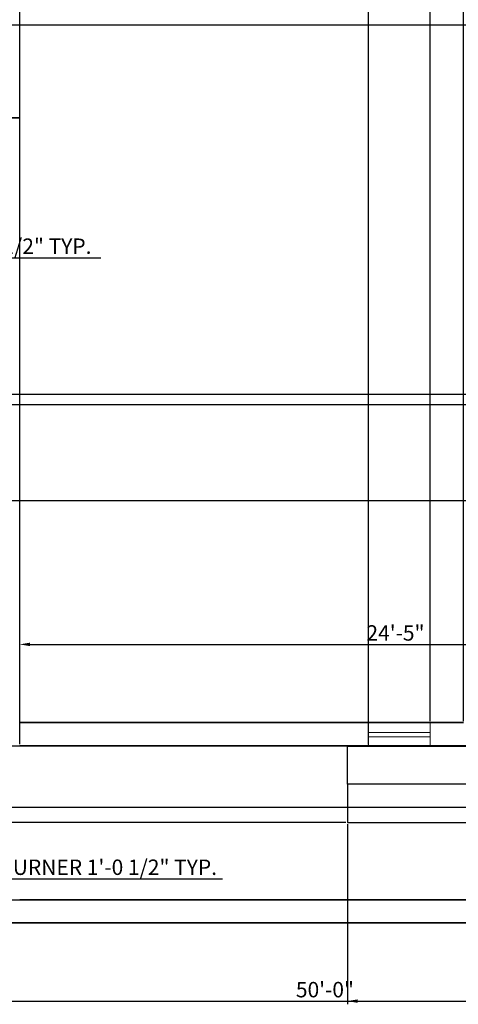
# Model space of a CAD drawing. Units: inches. Extents: x 1973 to 2661, y 1730 to 2412.
# Tile 2 of 5: x 2197 to 2368, y 1734 to 2117. Entities that reach past the tile are written whole.
import ezdxf

# ---------------------------------------------------------------- set-up
doc = ezdxf.new("R2010")
doc.units = ezdxf.units.IN
for name, color, linetype, lineweight in [('A-ANNO-DIMS', 2, 'Continuous', 18), ('A-FLOR-STRS', 7, 'Continuous', 25), ('A-GLAZ', 4, 'Continuous', 18), ('A-WALL', 7, 'Continuous', 35)]:
    doc.layers.add(name, color=color, linetype=linetype, lineweight=lineweight)
doc.styles.get("Standard").update_dxf_attribs({"font": 'arial.ttf'})
doc.dimstyles.new('ISO-25', dxfattribs={"dimtxt": 6, "dimasz": 4, "dimexe": 1.25, "dimexo": 0.625, "dimtad": 1, "dimdec": 0, "dimrnd": 6, "dimlunit": 3, "dimtxsty": 'Standard', "dimcen": 2.5, "dimadec": 0, "dimazin": 0, "dimtfac": 1, "dimtdec": 0, "dimtmove": 0, "dimatfit": 3, "dimfxl": 1, "dimarcsym": 0})

# ---------------------------------------------------------------- blocks, each defined once
blk = doc.blocks.new('*D16')
at = {"layer": 'A-ANNO-DIMS', "color": 0, "lineweight": -2, "transparency": 16777216}
for p, q in [((2092.18, 2025.82), (2092.18, 2023.31)), ((2096.18, 2024.56), (2100.77, 2024.56)), ((2104.77, 2025.82), (2104.77, 2023.31)), ((2104.77, 2024.56), (2228.74, 2024.56))]:
    blk.add_line(p, q, dxfattribs=at)
at = {"layer": 'A-ANNO-DIMS', "color": 0, "transparency": 16777216}
for points in [[(2096.18, 2025.23), (2096.18, 2023.89), (2092.18, 2024.56)], [(2100.77, 2025.23), (2100.77, 2023.89), (2104.77, 2024.56)]]:
    blk.add_solid(points, dxfattribs=at)
at = {"layer": 'Defpoints', "color": 0, "transparency": 16777216}
for p in [(2092.18, 2026.45), (2104.77, 2026.45), (2104.77, 2024.56)]:
    blk.add_point(p, dxfattribs=at)
at = {"layer": 'A-ANNO-DIMS', "color": 0, "transparency": 16777216, "insert": (2168.76, 2028.29), "char_height": 6, "attachment_point": 5}
blk.add_mtext('PLACE SETTING 1\'-0 1/2" TYP.', dxfattribs=at)
blk = doc.blocks.new('*D28')
at = {"layer": 'A-ANNO-DIMS', "color": 0, "lineweight": -2, "transparency": 16777216}
for p, q in [((2170.36, 1783.74), (2170.36, 1781.24)), ((2174.36, 1782.49), (2178.84, 1782.49)), ((2182.84, 1783.74), (2182.84, 1781.24)), ((2182.84, 1782.49), (2276.1, 1782.49))]:
    blk.add_line(p, q, dxfattribs=at)
at = {"layer": 'A-ANNO-DIMS', "color": 0, "transparency": 16777216}
for points in [[(2174.36, 1783.16), (2174.36, 1781.83), (2170.36, 1782.49)], [(2178.84, 1783.16), (2178.84, 1781.83), (2182.84, 1782.49)]]:
    blk.add_solid(points, dxfattribs=at)
at = {"layer": 'Defpoints', "color": 0, "transparency": 16777216}
for p in [(2170.36, 1784.36), (2182.84, 1784.36), (2182.84, 1782.49)]:
    blk.add_point(p, dxfattribs=at)
at = {"layer": 'A-ANNO-DIMS', "color": 0, "transparency": 16777216, "insert": (2231.47, 1786.22), "char_height": 6, "attachment_point": 5}
blk.add_mtext('BURNER 1\'-0 1/2" TYP.', dxfattribs=at)
blk = doc.blocks.new('*D30')
at = {"layer": 'A-ANNO-DIMS', "color": 0, "lineweight": -2, "transparency": 16777216}
for p, q in [((2016.04, 1764.73), (2016.04, 1733.57)), ((2616.04, 1764.73), (2616.04, 1733.57)), ((2020.04, 1734.82), (2612.04, 1734.82))]:
    blk.add_line(p, q, dxfattribs=at)
at = {"layer": 'A-ANNO-DIMS', "color": 0, "transparency": 16777216}
for points in [[(2020.04, 1735.49), (2020.04, 1734.15), (2016.04, 1734.82)], [(2612.04, 1735.49), (2612.04, 1734.15), (2616.04, 1734.82)]]:
    blk.add_solid(points, dxfattribs=at)
at = {"layer": 'Defpoints', "color": 0, "transparency": 16777216}
for p in [(2016.04, 1765.35), (2616.04, 1765.35), (2616.04, 1734.82)]:
    blk.add_point(p, dxfattribs=at)
at = {"layer": 'A-ANNO-DIMS', "color": 0, "transparency": 16777216, "insert": (2316.04, 1738.51), "char_height": 6, "attachment_point": 5}
blk.add_mtext('50\'-0"', dxfattribs=at)
blk = doc.blocks.new('*D53')
at = {"layer": 'A-ANNO-DIMS', "color": 0, "lineweight": -2, "transparency": 16777216}
for p, q in [((2197.04, 1843.98), (2197.04, 1875.1)), ((2201.04, 1873.85), (2486.04, 1873.85)), ((2490.04, 1843.98), (2490.04, 1875.1))]:
    blk.add_line(p, q, dxfattribs=at)
at = {"layer": 'A-ANNO-DIMS', "color": 0, "transparency": 16777216}
for points in [[(2201.04, 1874.52), (2201.04, 1873.18), (2197.04, 1873.85)], [(2486.04, 1874.52), (2486.04, 1873.18), (2490.04, 1873.85)]]:
    blk.add_solid(points, dxfattribs=at)
at = {"layer": 'Defpoints', "color": 0, "transparency": 16777216}
for p in [(2490.04, 1873.85), (2197.04, 1843.35), (2490.04, 1843.35)]:
    blk.add_point(p, dxfattribs=at)
at = {"layer": 'A-ANNO-DIMS', "color": 0, "transparency": 16777216, "insert": (2343.54, 1877.54), "char_height": 6, "attachment_point": 5}
blk.add_mtext('24\'-5"', dxfattribs=at)
blk = doc.blocks.new('*D54')
at = {"layer": 'A-ANNO-DIMS', "color": 0, "lineweight": -2, "transparency": 16777216}
for p, q in [((2197.04, 1834.98), (2197.04, 2397.1)), ((2201.04, 2395.85), (2329.03, 2395.85)), ((2333.03, 1834.87), (2333.03, 2397.1))]:
    blk.add_line(p, q, dxfattribs=at)
at = {"layer": 'A-ANNO-DIMS', "color": 0, "transparency": 16777216}
for points in [[(2201.04, 2396.52), (2201.04, 2395.18), (2197.04, 2395.85)], [(2329.03, 2396.52), (2329.03, 2395.18), (2333.03, 2395.85)]]:
    blk.add_solid(points, dxfattribs=at)
at = {"layer": 'Defpoints', "color": 0, "transparency": 16777216}
for p in [(2333.03, 2395.85), (2197.04, 1834.35), (2333.03, 1834.25)]:
    blk.add_point(p, dxfattribs=at)
at = {"layer": 'A-ANNO-DIMS', "color": 0, "transparency": 16777216, "insert": (2265.03, 2399.49), "char_height": 6, "attachment_point": 5}
blk.add_mtext('11\'-4"', dxfattribs=at)
blk = doc.blocks.new('*D57')
at = {"layer": 'A-ANNO-DIMS', "color": 0, "lineweight": -2, "transparency": 16777216}
for p, q in [((2193.67, 1810.35), (2647.79, 1810.35)), ((2646.54, 1778.35), (2646.54, 1806.35)), ((2193.67, 1774.35), (2647.79, 1774.35))]:
    blk.add_line(p, q, dxfattribs=at)
at = {"layer": 'A-ANNO-DIMS', "color": 0, "transparency": 16777216}
for points in [[(2645.88, 1806.35), (2647.21, 1806.35), (2646.54, 1810.35)], [(2645.88, 1778.35), (2647.21, 1778.35), (2646.54, 1774.35)]]:
    blk.add_solid(points, dxfattribs=at)
at = {"layer": 'Defpoints', "color": 0, "transparency": 16777216}
for p in [(2193.04, 1810.35), (2646.54, 1810.35), (2193.04, 1774.35)]:
    blk.add_point(p, dxfattribs=at)
at = {"layer": 'A-ANNO-DIMS', "color": 0, "transparency": 16777216, "insert": (2642.85, 1792.35), "char_height": 6, "attachment_point": 5, "rotation": 90}
blk.add_mtext('3\'-0"', dxfattribs=at)
blk = doc.blocks.new('*D59')
at = {"layer": 'A-ANNO-DIMS', "color": 0, "lineweight": -2, "transparency": 16777216}
for p, q in [((2193.67, 2115.35), (2647.79, 2115.35)), ((2646.54, 1975.35), (2646.54, 2111.35)), ((2193.67, 1971.35), (2647.79, 1971.35))]:
    blk.add_line(p, q, dxfattribs=at)
at = {"layer": 'A-ANNO-DIMS', "color": 0, "transparency": 16777216}
for points in [[(2645.88, 2111.35), (2647.21, 2111.35), (2646.54, 2115.35)], [(2645.88, 1975.35), (2647.21, 1975.35), (2646.54, 1971.35)]]:
    blk.add_solid(points, dxfattribs=at)
at = {"layer": 'Defpoints', "color": 0, "transparency": 16777216}
for p in [(2193.04, 2115.35), (2646.54, 2115.35), (2193.04, 1971.35)]:
    blk.add_point(p, dxfattribs=at)
at = {"layer": 'A-ANNO-DIMS', "color": 0, "transparency": 16777216, "insert": (2642.85, 2043.35), "char_height": 6, "attachment_point": 5, "rotation": 90}
blk.add_mtext('12\'-0"', dxfattribs=at)
blk = doc.blocks.new('*D64')
at = {"layer": 'A-ANNO-DIMS', "color": 0, "lineweight": -2, "transparency": 16777216}
for p, q in [((2324.17, 1834.25), (1984.22, 1834.25)), ((1985.47, 1808.45), (1985.47, 1830.25)), ((2324.17, 1804.45), (1984.22, 1804.45))]:
    blk.add_line(p, q, dxfattribs=at)
at = {"layer": 'A-ANNO-DIMS', "color": 0, "transparency": 16777216}
for points in [[(1984.81, 1830.25), (1986.14, 1830.25), (1985.47, 1834.25)], [(1984.81, 1808.45), (1986.14, 1808.45), (1985.47, 1804.45)]]:
    blk.add_solid(points, dxfattribs=at)
at = {"layer": 'Defpoints', "color": 0, "transparency": 16777216}
for p in [(1985.47, 1834.25), (2324.79, 1834.25), (2324.79, 1804.45)]:
    blk.add_point(p, dxfattribs=at)
at = {"layer": 'A-ANNO-DIMS', "color": 0, "transparency": 16777216, "insert": (1981.79, 1819.35), "char_height": 6, "attachment_point": 5, "rotation": 90}
blk.add_mtext('2\'-6"', dxfattribs=at)
blk = doc.blocks.new('*D65')
at = {"layer": 'A-ANNO-DIMS', "color": 0, "lineweight": -2, "transparency": 16777216}
for p, q in [((2324.79, 1803.83), (2324.79, 1733.57)), ((2485.69, 1803.83), (2485.69, 1733.57)), ((2328.79, 1734.82), (2481.69, 1734.82))]:
    blk.add_line(p, q, dxfattribs=at)
at = {"layer": 'A-ANNO-DIMS', "color": 0, "transparency": 16777216}
for points in [[(2328.79, 1735.49), (2328.79, 1734.15), (2324.79, 1734.82)], [(2481.69, 1735.49), (2481.69, 1734.15), (2485.69, 1734.82)]]:
    blk.add_solid(points, dxfattribs=at)
at = {"layer": 'Defpoints', "color": 0, "transparency": 16777216}
for p in [(2324.79, 1804.45), (2485.69, 1804.45), (2485.69, 1734.82)]:
    blk.add_point(p, dxfattribs=at)
at = {"layer": 'A-ANNO-DIMS', "color": 0, "transparency": 16777216, "insert": (2405.24, 1738.51), "char_height": 6, "attachment_point": 5}
blk.add_mtext('13\'-5"', dxfattribs=at)
blk = doc.blocks.new('*D66')
at = {"layer": 'A-ANNO-DIMS', "color": 0, "lineweight": -2, "transparency": 16777216}
for p, q in [((2333.03, 1843.98), (2333.03, 2397.1)), ((2337.03, 2395.85), (2353.02, 2395.85)), ((2357.02, 1843.98), (2357.02, 2397.1))]:
    blk.add_line(p, q, dxfattribs=at)
at = {"layer": 'A-ANNO-DIMS', "color": 0, "transparency": 16777216}
for points in [[(2337.03, 2396.52), (2337.03, 2395.18), (2333.03, 2395.85)], [(2353.02, 2396.52), (2353.02, 2395.18), (2357.02, 2395.85)]]:
    blk.add_solid(points, dxfattribs=at)
at = {"layer": 'Defpoints', "color": 0, "transparency": 16777216}
for p in [(2357.02, 2395.85), (2333.03, 1843.35), (2357.02, 1843.35)]:
    blk.add_point(p, dxfattribs=at)
at = {"layer": 'A-ANNO-DIMS', "color": 0, "transparency": 16777216, "insert": (2345.02, 2399.54), "char_height": 6, "attachment_point": 5}
blk.add_mtext('2\'-0"', dxfattribs=at)
blk = doc.blocks.new('*D69')
at = {"layer": 'A-ANNO-DIMS', "color": 0, "lineweight": -2, "transparency": 16777216}
for p, q in [((2357.02, 1843.98), (2357.02, 2397.1)), ((2361.02, 2395.85), (2366.04, 2395.85)), ((2370.04, 1843.98), (2370.04, 2397.1)), ((2370.04, 2395.85), (2390.68, 2395.85))]:
    blk.add_line(p, q, dxfattribs=at)
at = {"layer": 'A-ANNO-DIMS', "color": 0, "transparency": 16777216}
for points in [[(2361.02, 2396.52), (2361.02, 2395.18), (2357.02, 2395.85)], [(2366.04, 2396.52), (2366.04, 2395.18), (2370.04, 2395.85)]]:
    blk.add_solid(points, dxfattribs=at)
at = {"layer": 'Defpoints', "color": 0, "transparency": 16777216}
for p in [(2370.04, 2395.85), (2357.02, 1843.35), (2370.04, 1843.35)]:
    blk.add_point(p, dxfattribs=at)
at = {"layer": 'A-ANNO-DIMS', "color": 0, "transparency": 16777216, "insert": (2382.36, 2399.49), "char_height": 6, "attachment_point": 5}
blk.add_mtext('1\'-1"', dxfattribs=at)
blk = doc.blocks.new('*D73')
at = {"layer": 'A-ANNO-DIMS', "color": 0, "lineweight": -2, "transparency": 16777216}
for p, q in [((2066.89, 1967.35), (2647.79, 1967.35)), ((2646.54, 1933.97), (2646.54, 1963.35)), ((2066.89, 1929.97), (2647.79, 1929.97))]:
    blk.add_line(p, q, dxfattribs=at)
at = {"layer": 'A-ANNO-DIMS', "color": 0, "transparency": 16777216}
for points in [[(2645.88, 1963.35), (2647.21, 1963.35), (2646.54, 1967.35)], [(2645.88, 1933.97), (2647.21, 1933.97), (2646.54, 1929.97)]]:
    blk.add_solid(points, dxfattribs=at)
at = {"layer": 'Defpoints', "color": 0, "transparency": 16777216}
for p in [(2066.26, 1967.35), (2646.54, 1967.35), (2066.26, 1929.97)]:
    blk.add_point(p, dxfattribs=at)
at = {"layer": 'A-ANNO-DIMS', "color": 0, "transparency": 16777216, "insert": (2642.81, 1948.66), "char_height": 6, "attachment_point": 5, "rotation": 90}
blk.add_mtext('3\'-1 1/2"', dxfattribs=at)

msp = doc.modelspace()

# ---------------------------------------------------------------- linework, layer by layer
at = {"layer": 'A-FLOR-STRS'}
for p, q in [((2324.79, 1834.25), (2485.69, 1834.25)), ((2324.79, 1819.35), (2324.79, 1834.25)), ((2324.79, 1834.25), (2333.03, 1834.25)), ((2485.69, 1819.35), (2324.79, 1819.35)), ((2485.69, 1819.35), (2324.79, 1819.35)), ((2324.79, 1819.35), (2324.79, 1804.45)), ((2324.79, 1804.45), (2485.69, 1804.45))]:
    msp.add_line(p, q, dxfattribs=at)
at = {"layer": 'A-GLAZ'}
for p, q in [((2333.03, 1834.25), (2333.03, 1843.35)), ((2333.03, 1843.35), (2357.02, 1843.35)), ((2357.02, 1843.35), (2357.02, 1834.35)), ((2333.03, 1837.89), (2333.03, 1839.49)), ((2333.03, 1839.49), (2357.02, 1839.49)), ((2357.02, 1837.89), (2333.03, 1837.89)), ((2357.02, 1834.35), (2357.02, 1837.89))]:
    msp.add_line(p, q, dxfattribs=at)
at = {"layer": 'A-WALL'}
for p, q in [((2193.04, 2079.16), (2197.09, 2079.1)), ((2370.04, 1843.35), (2197.04, 1843.35)), ((2197.04, 1834.35), (2499.04, 1834.35)), ((2197.04, 1774.35), (2607.04, 1774.35)), ((2616.04, 1765.35), (2016.04, 1765.35))]:
    msp.add_line(p, q, dxfattribs=at)

# ---------------------------------------------------------------- dimensions: what is measured, and where the dimension line sits
at = {"layer": 'A-ANNO-DIMS'}
for base, p1, p2, picture, middle in [((2333.03, 2395.85), (2197.04, 1834.35), (2333.03, 1834.25), '*D54', (2265.03, 2399.49)), ((2357.02, 2395.85), (2333.03, 1843.35), (2357.02, 1843.35), '*D66', (2345.02, 2399.54)), ((2370.04, 2395.85), (2357.02, 1843.35), (2370.04, 1843.35), '*D69', (2382.36, 2399.49)), ((2490.04, 1873.85), (2197.04, 1843.35), (2490.04, 1843.35), '*D53', (2343.54, 1877.54)), ((2485.69, 1734.82), (2324.79, 1804.45), (2485.69, 1804.45), '*D65', (2405.24, 1738.51)), ((2616.04, 1734.82), (2016.04, 1765.35), (2616.04, 1765.35), '*D30', (2316.04, 1738.51))]:
    dim = msp.add_linear_dim(base=base, p1=p1, p2=p2, dimstyle='ISO-25', override={"dimdec": 1, "dimlfac": 1, "dimrnd": 0, "dimzin": 1, "dimdsep": 46, "dimlunit": 4, "dimfrac": 2}, dxfattribs=at)
    dim.commit()
    dim.dimension.update_dxf_attribs({"geometry": picture, "text_midpoint": middle})
for base, p1, p2, picture, middle in [((2646.54, 2115.35), (2193.04, 1971.35), (2193.04, 2115.35), '*D59', (2642.85, 2043.35)), ((2646.54, 1967.35), (2066.26, 1929.97), (2066.26, 1967.35), '*D73', (2642.81, 1948.66)), ((1985.47, 1834.25), (2324.79, 1804.45), (2324.79, 1834.25), '*D64', (1981.79, 1819.35)), ((2646.54, 1810.35), (2193.04, 1774.35), (2193.04, 1810.35), '*D57', (2642.85, 1792.35))]:
    dim = msp.add_linear_dim(base=base, p1=p1, p2=p2, angle=90, dimstyle='ISO-25', override={"dimdec": 1, "dimlfac": 1, "dimrnd": 0, "dimzin": 1, "dimdsep": 46, "dimlunit": 4, "dimfrac": 2}, dxfattribs=at)
    dim.commit()
    dim.dimension.update_dxf_attribs({"geometry": picture, "text_midpoint": middle})
for base, p1, p2, text, picture, middle in [((2104.77, 2024.56), (2092.18, 2026.45), (2104.77, 2026.45), 'PLACE SETTING <> TYP.', '*D16', (2168.76, 2028.29)), ((2182.84, 1782.49), (2170.36, 1784.36), (2182.84, 1784.36), 'BURNER <> TYP.', '*D28', (2231.47, 1786.22))]:
    dim = msp.add_linear_dim(base=base, p1=p1, p2=p2, text=text, dimstyle='ISO-25', override={"dimdec": 1, "dimlfac": 1, "dimrnd": 0, "dimzin": 1, "dimdsep": 46, "dimlunit": 4, "dimfrac": 2}, dxfattribs=at)
    dim.commit()
    dim.dimension.update_dxf_attribs({"geometry": picture, "text_midpoint": middle})

doc.saveas('drawing.dxf')
